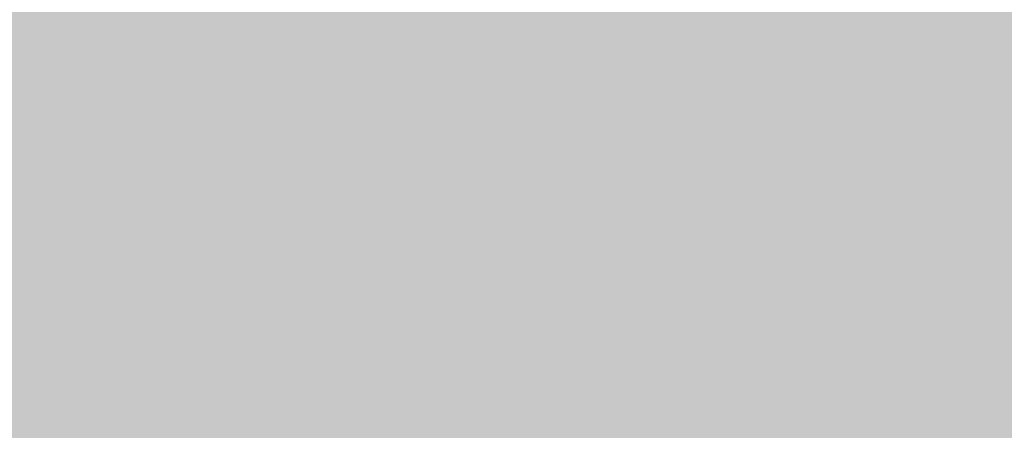
# Model space of a CAD drawing. Units: feet. Extents: x 3168 to 4724, y 827 to 1477.
# Tile 150 of 256: x 3301.1638 to 3301.19778, y 1099.00068 to 1099.01485. Entities that reach past the tile are written whole.
import ezdxf

# ---------------------------------------------------------------- set-up
doc = ezdxf.new("R2010")
doc.units = ezdxf.units.FT
doc.layers.add('A-ELEV', color=7, linetype='Continuous', lineweight=35)
doc.layers.add('A-ELEV-PATT', color=8, linetype='Continuous', lineweight=13)

msp = doc.modelspace()

# ---------------------------------------------------------------- hatches: boundary and pattern name
at = {"layer": 'A-ELEV-PATT'}
h = msp.add_hatch(color=256, dxfattribs=at)
h.dxf.hatch_style = 1
edge = h.paths.add_edge_path()
edge.add_ellipse((3552.905762, 979.220141), major_axis=(36.744924, 0), ratio=0.484848485, start_angle=0, end_angle=360)
edge = h.paths.add_edge_path()
edge.add_ellipse((3559.891637, 929.252282), major_axis=(36.744924, 0), ratio=0.484848485, start_angle=0, end_angle=360)
edge = h.paths.add_edge_path()
edge.add_line((3299.31681, 1198.606081), (3479.916714, 1198.606081))
edge.add_line((3479.916714, 1198.606081), (3479.916714, 1209.86857))
edge.add_spline(control_points=[(3479.916714, 1209.86857), (3464.301157, 1209.86857), (3448.685601, 1209.86857), (3410.949139, 1209.86857), (3388.828234, 1209.86857), (3355.646876, 1209.86857), (3344.586423, 1209.86857), (3327.995745, 1209.86857), (3322.465518, 1209.86857), (3314.170179, 1209.86857), (3311.405066, 1209.86857), (3307.257396, 1209.86857), (3305.874839, 1209.86857), (3303.801005, 1209.86857), (3303.109726, 1209.86857), (3302.072809, 1209.86857), (3301.72717, 1209.86857), (3301.208711, 1209.86857), (3301.035891, 1209.86857), (3300.776662, 1209.86857), (3300.690252, 1209.86857), (3300.560638, 1209.86857), (3300.517433, 1209.86857), (3300.452625, 1209.86857), (3300.431023, 1209.86857), (3300.398619, 1209.86857), (3300.387818, 1209.86857), (3300.366216, 1209.86857), (3300.345676, 1209.86857), (3300.345548, 1209.86857), (3300.345505, 1209.86857), (3300.343304, 1209.86857), (3300.341146, 1209.868571), (3300.337909, 1209.868571), (3300.33683, 1209.868572), (3300.333942, 1209.868573), (3300.332133, 1209.868574), (3300.325515, 1209.868577), (3300.320706, 1209.868581), (3300.310925, 1209.868592), (3300.305952, 1209.868598), (3300.290511, 1209.868623), (3300.280045, 1209.868646), (3300.232425, 1209.868777), (3300.195298, 1209.868954), (3299.951068, 1209.870608), (3299.744824, 1209.874326), (3299.436827, 1209.883257), (3299.334389, 1209.886792), (3299.181079, 1209.89292), (3299.130033, 1209.895099), (3298.652217, 1209.916801), (3298.22946, 1209.945718), (3297.601631, 1210.002367), (3297.393404, 1210.023464), (3297.082652, 1210.058309), (3296.979332, 1210.070458), (3296.292954, 1210.154861), (3295.718148, 1210.243356), (3294.868717, 1210.39885), (3294.5877, 1210.454478), (3294.169341, 1210.543349), (3294.030415, 1210.573878), (3291.707149, 1211.1012), (3289.65359, 1211.813435), (3285.776259, 1213.563988), (3283.95141, 1214.603478), (3280.512159, 1216.98008), (3278.897241, 1218.317592), (3276.379914, 1220.829489), (3275.416042, 1221.917738), (3274.039342, 1223.7077), (3273.581043, 1224.349535), (3273.143228, 1225.016316)], knot_values=[39.119033, 39.119033, 39.119033, 39.119033, 39.286353, 39.286353, 39.523379, 39.523379, 39.641892, 39.641892, 39.701148, 39.701148, 39.730777, 39.730777, 39.745591, 39.745591, 39.752998, 39.752998, 39.756701, 39.756701, 39.758553, 39.758553, 39.759479, 39.759479, 39.759942, 39.759942, 39.760173, 39.760173, 39.760289, 39.760289, 39.760405, 39.760405, 39.760463, 39.760463, 39.763389, 39.763389, 39.764851, 39.764851, 39.767304, 39.767304, 39.773825, 39.773825, 39.78057, 39.78057, 39.79477, 39.79477, 39.845194, 39.845194, 40.126715, 40.126715, 40.267476, 40.267476, 40.337856, 40.337856, 40.927023, 40.927023, 41.221606, 41.221606, 41.368898, 41.368898, 42.202622, 42.202622, 42.619485, 42.619485, 42.827916, 42.827916, 46.118323, 46.118323, 49.408731, 49.408731, 52.699139, 52.699139, 54.927489, 54.927489, 56.104228, 56.104228, 56.104228, 56.104228], weights=[1, 1, 1, 1, 1, 1, 1, 1, 1, 1, 1, 1, 1, 1, 1, 1, 1, 1, 1, 1, 1, 1, 1, 1, 1, 1, 1, 1, 1, 1, 1, 1, 1, 1, 1, 1, 1, 1, 1, 1, 1, 1, 1, 1, 1, 1, 1, 1, 1, 1, 1, 1, 1, 1, 1, 1, 1, 1, 1, 1, 1, 1, 1, 1, 1, 1, 1, 1, 1, 1, 1, 1, 1, 1], degree=3, periodic=0)
edge.add_line((3273.143228, 1225.016316), (3273.143228, 1099.016316))
edge.add_line((3273.143228, 1099.016316), (3299.31681, 1099.016316))
edge.add_line((3299.31681, 1099.016316), (3299.31681, 1198.606081))
edge = h.paths.add_edge_path()
edge.add_line((3304.758443, 1324.15806), (3479.916714, 1324.15806))
edge.add_line((3479.916714, 1324.15806), (3479.916714, 1335.714618))
edge.add_line((3479.916714, 1335.714618), (3269.161628, 1335.714618))
edge.add_spline(control_points=[(3269.161628, 1335.714618), (3264.024231, 1335.714618), (3258.364118, 1328.958189), (3259.264311, 1323.900274)], knot_values=[0, 0, 0, 0, 15.412191, 15.412191, 15.412191, 15.412191], degree=3, periodic=0)
edge.add_line((3259.264311, 1323.900274), (3265.516849, 1288.769135))
edge.add_line((3265.516849, 1288.769135), (3275.265103, 1261.545626))
edge.add_line((3275.265103, 1261.545626), (3304.758443, 1261.545626))
edge.add_line((3304.758443, 1261.545626), (3304.758443, 1324.15806))
h = msp.add_hatch(color=256, dxfattribs=at)
h.dxf.hatch_style = 1
h.paths.add_polyline_path([(3384.525247, 1099.016316), (3335.029168, 1099.016316), (3299.31681, 1099.016316), (3273.143228, 1099.016316), (3217.565364, 1099.016316), (3168.069285, 827.11626), (3335.029168, 827.11626)])

# ---------------------------------------------------------------- linework, layer by layer
at = {"layer": 'A-ELEV'}
msp.add_open_spline([(3808.5202, 1099.016316), (3808.5202, 1141.413235), (3808.5202, 1183.810154), (3808.5202, 1226.635324), (3808.5202, 1227.063576), (3808.5202, 1227.491828), (3811.491871, 1248.994673), (3814.463542, 1270.497518), (3817.46523, 1292.217564), (3817.495247, 1292.434764), (3817.525264, 1292.651964), (3817.572801, 1310.106748), (3817.620339, 1327.561532), (3817.667877, 1345.016316), (3817.667877, 1345.457962), (3817.667877, 1345.899608), (3817.667877, 1346.456047), (3817.667877, 1346.57084), (3817.667877, 1346.752887), (3817.667877, 1346.820142), (3817.667877, 1346.93487), (3817.667877, 1346.982345), (3817.667877, 1347.038587), (3817.667877, 1347.047356), (3817.667877, 1347.073661), (3817.667877, 1347.059303), (3817.667877, 1347.061545), (3817.667876, 1347.062667), (3817.667875, 1347.066031), (3817.667874, 1347.068274), (3817.66787, 1347.075001), (3817.667866, 1347.079486), (3817.667849, 1347.092937), (3817.667833, 1347.101902), (3817.667766, 1347.12879), (3817.667699, 1347.146705), (3817.667432, 1347.200421), (3817.667165, 1347.236192), (3817.6661, 1347.343385), (3817.665038, 1347.414686), (3817.660812, 1347.628095), (3817.656608, 1347.769708), (3817.63997, 1348.192487), (3817.623509, 1348.471586), (3817.559094, 1349.300067), (3817.496121, 1349.840588), (3817.255432, 1351.424156), (3817.026318, 1352.428785), (3816.306871, 1354.888914), (3815.743745, 1356.268727), (3814.463959, 1358.81921), (3813.746413, 1359.990968), (3812.195838, 1362.172343), (3811.362245, 1363.182124), (3809.588836, 1365.069009), (3808.648816, 1365.946105), (3806.654262, 1367.579616), (3805.599702, 1368.336154), (3803.352891, 1369.722327), (3802.160535, 1370.352386), (3799.600813, 1371.453586), (3798.232688, 1371.925481), (3795.280084, 1372.634624), (3793.693148, 1372.872068), (3791.869441, 1372.92648), (3791.740861, 1372.92922), (3791.353371, 1372.934101), (3791.092707, 1372.932901), (3790.304116, 1372.915068), (3789.769543, 1372.884195), (3789.20919, 1372.830236), (3789.190622, 1372.828424), (3789.134892, 1372.822912), (3789.097705, 1372.819137), (3789.048445, 1372.814008), (3789.0364, 1372.812743), (3789.000256, 1372.808918), (3788.976147, 1372.806325), (3788.949405, 1372.803404), (3788.946786, 1372.803118), (3788.942567, 1372.802655), (3788.940967, 1372.80248), (3788.938572, 1372.802217), (3788.937777, 1372.802129), (3788.935391, 1372.801867), (3788.867535, 1372.794402), (3788.756866, 1372.782228), (3788.701532, 1372.776141), (3788.53553, 1372.75788), (3788.424861, 1372.745707), (3788.092856, 1372.709185), (3787.871519, 1372.684837), (3787.207509, 1372.611793), (3786.764835, 1372.563097), (3785.436814, 1372.417009), (3784.551467, 1372.319617), (3781.895425, 1372.027442), (3780.12473, 1371.832658), (3774.812646, 1371.248307), (3771.271256, 1370.858739), (3760.647088, 1369.690037), (3753.56431, 1368.910902), (3732.315973, 1366.573498), (3718.150416, 1365.015228), (3694.006758, 1362.359326), (3684.028657, 1361.261694), (3674.050557, 1360.164062), (3664.600662, 1360.164062), (3655.150767, 1360.164062), (3626.801081, 1360.164062), (3607.901291, 1360.164062), (3551.20192, 1360.164062), (3513.40234, 1360.164062), (3467.725182, 1360.164062), (3459.847604, 1360.164062), (3436.214873, 1360.164062), (3420.459718, 1360.164062), (3373.194255, 1360.164062), (3341.683946, 1360.164062), (3302.848162, 1360.164062), (3295.522686, 1360.164062), (3286.038292, 1360.164062), (3283.879372, 1360.164062), (3277.402613, 1360.164062), (3273.084773, 1360.164062), (3267.732851, 1360.164062), (3266.698768, 1360.164062), (3263.59652, 1360.164062), (3261.528355, 1360.164062), (3259.236943, 1360.164062), (3259.013697, 1360.164062), (3258.343958, 1360.164062), (3257.897466, 1360.164062), (3257.430998, 1360.164062), (3257.411022, 1360.164062), (3257.370573, 1360.164062), (3257.37547, 1360.164062), (3257.374598, 1360.164062), (3257.373937, 1360.164062), (3257.371956, 1360.164062), (3257.370635, 1360.164061), (3257.366673, 1360.16406), (3257.364032, 1360.164059), (3257.356109, 1360.164053), (3257.350828, 1360.164047), (3257.334987, 1360.164023), (3257.32443, 1360.163998), (3257.292769, 1360.163899), (3257.271676, 1360.163799), (3257.208439, 1360.163398), (3257.166337, 1360.162995), (3257.040206, 1360.161388), (3256.956349, 1360.159783), (3256.705504, 1360.153393), (3256.53924, 1360.147036), (3256.04357, 1360.121916), (3255.717296, 1360.097102), (3254.752446, 1360.000481), (3254.127968, 1359.906513), (3252.180067, 1359.525332), (3250.941574, 1359.143991), (3248.670175, 1358.24329), (3247.635739, 1357.723834), (3245.732632, 1356.603471), (3244.863388, 1356.00206), (3243.253108, 1354.742865), (3242.511972, 1354.084731), (3240.751052, 1352.344781), (3239.800961, 1351.229574), (3238.087769, 1348.87244), (3237.324685, 1347.630355), (3235.98251, 1344.971632), (3235.402205, 1343.554907), (3234.591081, 1340.815458), (3234.310882, 1339.54355), (3233.97649, 1336.802561), (3233.922113, 1335.330877), (3234.148916, 1332.591269), (3234.349529, 1331.367201), (3234.719893, 1329.999367), (3234.752423, 1329.883362), (3234.853619, 1329.534797), (3234.925892, 1329.301685), (3235.024836, 1329.002552), (3235.046924, 1328.936928), (3235.077639, 1328.847239), (3235.085924, 1328.823198), (3235.110939, 1328.751064), (3235.127828, 1328.702962), (3235.147992, 1328.646242), (3235.151059, 1328.637632), (3235.156096, 1328.623526), (3235.158061, 1328.61803), (3235.160209, 1328.61203), (3235.165612, 1328.596943), (3235.180099, 1328.556486), (3235.190263, 1328.528101), (3235.220756, 1328.442946), (3235.241084, 1328.386176), (3235.302069, 1328.215865), (3235.342726, 1328.102325), (3235.464696, 1327.761704), (3235.54601, 1327.534623), (3235.78995, 1326.853381), (3235.952577, 1326.39922), (3236.440459, 1325.036736), (3236.765713, 1324.128414), (3237.741475, 1321.403446), (3238.391983, 1319.586801), (3240.343508, 1314.136866), (3241.644525, 1310.503576), (3245.547574, 1299.603706), (3248.149607, 1292.337126), (3255.955706, 1270.537385), (3261.159772, 1256.004225), (3267.387618, 1238.612001), (3268.411397, 1235.752937), (3269.510378, 1232.683864), (3269.585579, 1232.473854), (3269.706612, 1232.135851), (3269.752444, 1232.007857), (3269.827329, 1231.79873), (3269.856382, 1231.717595), (3269.906325, 1231.578122), (3269.927215, 1231.519782), (3269.972468, 1231.393406), (3269.996831, 1231.325368), (3270.026503, 1231.242506), (3270.031811, 1231.227681), (3270.040282, 1231.204024), (3270.039224, 1231.206979), (3270.039359, 1231.206601), (3270.039427, 1231.206412), (3270.03963, 1231.205846), (3270.039765, 1231.205468), (3270.040171, 1231.204335), (3270.040442, 1231.203579), (3270.041254, 1231.201313), (3270.041796, 1231.199802), (3270.04342, 1231.195269), (3270.044504, 1231.192248), (3270.047756, 1231.183185), (3270.049926, 1231.177145), (3270.056442, 1231.159028), (3270.060793, 1231.146957), (3270.073867, 1231.110761), (3270.082613, 1231.086656), (3270.108936, 1231.014413), (3270.1266, 1230.96635), (3270.179934, 1230.822457), (3270.215947, 1230.726923), (3270.325323, 1230.441508), (3270.400026, 1230.252811), (3270.629249, 1229.691444), (3270.788883, 1229.323501), (3271.286488, 1228.238319), (3271.6431, 1227.539755), (3272.775859, 1225.515277), (3273.614169, 1224.260502), (3275.416042, 1221.917738), (3276.379914, 1220.829489), (3278.897241, 1218.317592), (3280.512159, 1216.98008), (3283.95141, 1214.603478), (3285.776259, 1213.563988), (3289.65359, 1211.813435), (3291.707149, 1211.1012), (3294.030415, 1210.573878), (3294.169341, 1210.543349), (3294.5877, 1210.454478), (3294.868717, 1210.39885), (3295.718148, 1210.243356), (3296.292954, 1210.154861), (3296.979332, 1210.070458), (3297.082652, 1210.058309), (3297.393404, 1210.023464), (3297.601631, 1210.002367), (3298.22946, 1209.945718), (3298.652217, 1209.916801), (3299.130033, 1209.895099), (3299.181079, 1209.89292), (3299.334389, 1209.886792), (3299.436827, 1209.883257), (3299.744824, 1209.874326), (3299.951068, 1209.870608), (3300.195298, 1209.868954), (3300.232425, 1209.868777), (3300.280045, 1209.868646), (3300.290511, 1209.868623), (3300.305952, 1209.868598), (3300.310925, 1209.868592), (3300.320706, 1209.868581), (3300.325515, 1209.868577), (3300.332133, 1209.868574), (3300.333942, 1209.868573), (3300.33683, 1209.868572), (3300.337909, 1209.868571), (3300.341146, 1209.868571), (3300.343304, 1209.86857), (3300.345505, 1209.86857), (3300.345548, 1209.86857), (3300.345676, 1209.86857), (3300.366216, 1209.86857), (3300.387818, 1209.86857), (3300.398619, 1209.86857), (3300.431023, 1209.86857), (3300.452625, 1209.86857), (3300.517433, 1209.86857), (3300.560638, 1209.86857), (3300.690252, 1209.86857), (3300.776662, 1209.86857), (3301.035891, 1209.86857), (3301.208711, 1209.86857), (3301.72717, 1209.86857), (3302.072809, 1209.86857), (3303.109726, 1209.86857), (3303.801005, 1209.86857), (3305.874839, 1209.86857), (3307.257396, 1209.86857), (3311.405066, 1209.86857), (3314.170179, 1209.86857), (3322.465518, 1209.86857), (3327.995745, 1209.86857), (3344.586423, 1209.86857), (3355.646876, 1209.86857), (3388.828234, 1209.86857), (3410.949139, 1209.86857), (3477.311855, 1209.86857), (3521.553665, 1209.86857), (3566.836184, 1209.86857), (3567.876892, 1209.86857), (3570.999017, 1209.86857), (3573.080433, 1209.86857), (3575.781396, 1209.86857), (3576.400943, 1209.86857), (3577.295821, 1209.86857), (3577.571152, 1209.86857), (3578.397146, 1209.86857), (3578.947808, 1209.86857), (3579.756491, 1209.86857), (3580.014511, 1209.86857), (3580.342737, 1209.86857), (3580.326865, 1209.86857), (3580.32717, 1209.86857), (3580.327323, 1209.86857), (3580.327781, 1209.86857), (3580.328086, 1209.86857), (3580.329002, 1209.86857), (3580.329613, 1209.86857), (3580.331445, 1209.86857), (3580.332667, 1209.86857), (3580.336332, 1209.868569), (3580.338775, 1209.868567), (3580.346107, 1209.868563), (3580.350995, 1209.868558), (3580.365663, 1209.86854), (3580.375445, 1209.868522), (3580.404801, 1209.868449), (3580.424386, 1209.868376), (3580.483183, 1209.868085), (3580.522437, 1209.867793), (3580.640361, 1209.866624), (3580.719195, 1209.865454), (3580.956315, 1209.860766), (3581.115222, 1209.85607), (3581.594164, 1209.83723), (3581.916419, 1209.818331), (3582.889947, 1209.742428), (3583.547986, 1209.666169), (3585.531827, 1209.360617), (3586.867216, 1209.053886), (3589.471545, 1208.252472), (3590.740241, 1207.757852), (3591.995451, 1207.158802), (3592.057809, 1207.12874), (3592.244242, 1207.037954), (3592.367676, 1206.976632), (3592.73528, 1206.790359), (3592.976752, 1206.663101), (3593.244539, 1206.516441), (3593.274731, 1206.499825), (3593.365115, 1206.449839), (3593.425113, 1206.416333), (3593.604314, 1206.315285), (3593.722725, 1206.247211), (3593.857212, 1206.168398), (3593.874362, 1206.158319), (3593.925741, 1206.128041), (3593.959899, 1206.107798), (3594.062086, 1206.046899), (3594.129827, 1206.006074), (3594.208436, 1205.958171), (3594.219683, 1205.951304), (3594.253391, 1205.930686), (3594.275819, 1205.916917), (3594.342972, 1205.875536), (3594.387563, 1205.847853), (3594.433616, 1205.81905), (3594.435256, 1205.818024), (3594.440175, 1205.814946), (3594.443453, 1205.812894), (3594.447123, 1205.810594), (3594.447516, 1205.810348), (3594.448695, 1205.80961), (3594.449481, 1205.809117), (3594.450366, 1205.808562), (3594.450466, 1205.8085), (3594.4506, 1205.808415), (3594.467399, 1205.797887), (3594.493269, 1205.781674), (3594.506204, 1205.773568), (3594.545008, 1205.749248), (3594.570878, 1205.733035), (3594.648487, 1205.684396), (3594.700226, 1205.651969), (3594.855444, 1205.554691), (3594.958922, 1205.489839), (3595.269357, 1205.295282), (3595.476314, 1205.165577), (3596.097185, 1204.776463), (3596.511099, 1204.517054), (3597.752841, 1203.738826), (3598.580669, 1203.220007), (3601.064152, 1201.663551), (3602.719807, 1200.625914), (3607.686774, 1197.513002), (3610.998085, 1195.437727), (3620.932018, 1189.211903), (3627.55464, 1185.061354), (3647.422507, 1172.609707), (3660.667751, 1164.308608), (3700.403484, 1139.405313), (3726.893973, 1122.803116), (3757.205715, 1103.806052), (3761.02697, 1101.411184), (3764.848224, 1099.016316), (3745.328271, 1099.016316), (3725.808319, 1099.016316), (3706.288366, 1099.016316), (3706.288366, 1108.453237), (3706.288366, 1117.890158), (3706.288366, 1127.327079), (3710.750754, 1127.327079), (3715.213143, 1127.327079), (3719.675531, 1127.327079)], degree=3, knots=[0, 0, 0, 0, 0.982037, 0.982037, 0.991957, 0.991957, 0.991957, 1.966522, 1.966522, 1.976367, 1.976367, 1.976367, 2.976367, 2.976367, 2.976367, 3.00169, 3.00169, 3.008272, 3.008272, 3.012129, 3.012129, 3.014851, 3.014851, 3.015353, 3.015353, 3.016359, 3.016359, 3.017365, 3.017365, 3.019376, 3.019376, 3.023398, 3.023398, 3.031442, 3.031442, 3.047531, 3.047531, 3.079708, 3.079708, 3.144063, 3.144063, 3.272772, 3.272772, 3.53019, 3.53019, 4.045026, 4.045026, 5.074698, 5.074698, 6.700878, 6.700878, 8.327058, 8.327058, 9.953238, 9.953238, 11.579418, 11.579418, 13.205598, 13.205598, 14.831778, 14.831778, 16.457958, 16.457958, 18.084138, 18.084138, 18.206872, 18.206872, 18.45234, 18.45234, 18.943275, 18.943275, 18.960093, 18.960093, 18.993729, 18.993729, 19.00461, 19.00461, 19.026374, 19.026374, 19.028737, 19.028737, 19.03018, 19.03018, 19.030897, 19.030897, 19.032332, 19.032332, 19.033766, 19.033766, 19.036636, 19.036636, 19.042374, 19.042374, 19.053851, 19.053851, 19.076805, 19.076805, 19.122714, 19.122714, 19.21453, 19.21453, 19.398163, 19.398163, 19.765429, 19.765429, 20.024128, 20.024128, 20.024128, 20.092031, 20.092031, 20.227836, 20.227836, 20.499446, 20.499446, 20.556051, 20.556051, 20.66926, 20.66926, 20.895678, 20.895678, 20.948316, 20.948316, 20.963829, 20.963829, 20.994855, 20.994855, 21.002285, 21.002285, 21.017146, 21.017146, 21.01875, 21.01875, 21.021959, 21.021959, 21.022102, 21.022102, 21.022249, 21.022249, 21.022708, 21.022708, 21.023627, 21.023627, 21.025464, 21.025464, 21.029138, 21.029138, 21.036486, 21.036486, 21.051183, 21.051183, 21.080575, 21.080575, 21.139361, 21.139361, 21.256932, 21.256932, 21.492073, 21.492073, 21.962356, 21.962356, 23.01002, 23.01002, 24.057684, 24.057684, 25.105348, 25.105348, 26.153011, 26.153011, 27.776787, 27.776787, 29.400562, 29.400562, 31.024337, 31.024337, 32.278801, 32.278801, 33.533265, 33.533265, 34.467568, 34.467568, 34.553971, 34.553971, 34.726776, 34.726776, 34.775309, 34.775309, 34.793079, 34.793079, 34.82862, 34.82862, 34.834979, 34.834979, 34.839039, 34.839039, 34.839411, 34.839411, 34.840285, 34.840285, 34.842034, 34.842034, 34.845531, 34.845531, 34.852525, 34.852525, 34.866512, 34.866512, 34.894488, 34.894488, 34.950439, 34.950439, 35.062342, 35.062342, 35.286147, 35.286147, 35.733758, 35.733758, 35.821815, 35.821815, 35.828283, 35.828283, 35.832225, 35.832225, 35.834724, 35.834724, 35.836521, 35.836521, 35.838617, 35.838617, 35.839073, 35.839073, 35.839345, 35.839345, 35.839617, 35.839617, 35.840161, 35.840161, 35.841249, 35.841249, 35.843425, 35.843425, 35.847778, 35.847778, 35.856482, 35.856482, 35.873891, 35.873891, 35.908709, 35.908709, 35.978345, 35.978345, 36.117617, 36.117617, 36.396161, 36.396161, 36.953248, 36.953248, 38.067423, 38.067423, 40.295772, 40.295772, 42.524122, 42.524122, 45.81453, 45.81453, 49.104937, 49.104937, 52.395345, 52.395345, 52.603776, 52.603776, 53.020639, 53.020639, 53.854363, 53.854363, 54.001655, 54.001655, 54.296238, 54.296238, 54.885405, 54.885405, 54.955785, 54.955785, 55.096546, 55.096546, 55.378067, 55.378067, 55.42849, 55.42849, 55.442691, 55.442691, 55.449436, 55.449436, 55.455957, 55.455957, 55.458409, 55.458409, 55.459872, 55.459872, 55.462798, 55.462798, 55.462856, 55.462856, 55.462972, 55.462972, 55.463088, 55.463088, 55.463319, 55.463319, 55.463782, 55.463782, 55.464708, 55.464708, 55.46656, 55.46656, 55.470263, 55.470263, 55.47767, 55.47767, 55.492484, 55.492484, 55.522112, 55.522112, 55.581369, 55.581369, 55.699882, 55.699882, 55.936907, 55.936907, 56.410959, 56.410959, 56.42211, 56.42211, 56.444413, 56.444413, 56.451051, 56.451051, 56.454001, 56.454001, 56.459901, 56.459901, 56.462666, 56.462666, 56.463418, 56.463418, 56.464171, 56.464171, 56.465675, 56.465675, 56.468684, 56.468684, 56.474702, 56.474702, 56.486738, 56.486738, 56.51081, 56.51081, 56.558955, 56.558955, 56.655243, 56.655243, 56.847821, 56.847821, 57.232975, 57.232975, 58.003284, 58.003284, 59.543901, 59.543901, 62.625137, 62.625137, 68.787607, 68.787607, 74.950078, 74.950078, 75.27336, 75.27336, 75.919923, 75.919923, 77.213051, 77.213051, 77.377769, 77.377769, 77.707206, 77.707206, 78.366079, 78.366079, 78.462532, 78.462532, 78.655436, 78.655436, 79.041245, 79.041245, 79.105735, 79.105735, 79.234714, 79.234714, 79.492672, 79.492672, 79.502197, 79.502197, 79.521249, 79.521249, 79.523534, 79.523534, 79.528103, 79.528103, 79.528682, 79.528682, 79.528885, 79.528885, 79.529089, 79.529089, 79.529495, 79.529495, 79.530308, 79.530308, 79.531935, 79.531935, 79.535187, 79.535187, 79.541693, 79.541693, 79.554704, 79.554704, 79.580725, 79.580725, 79.632769, 79.632769, 79.736856, 79.736856, 79.94503, 79.94503, 80.361377, 80.361377, 80.421435, 80.421435, 80.421435, 81.421435, 81.421435, 81.421435, 82.421435, 82.421435, 82.421435, 83.421435, 83.421435, 83.421435, 83.421435], dxfattribs=at)

doc.saveas('drawing.dxf')
